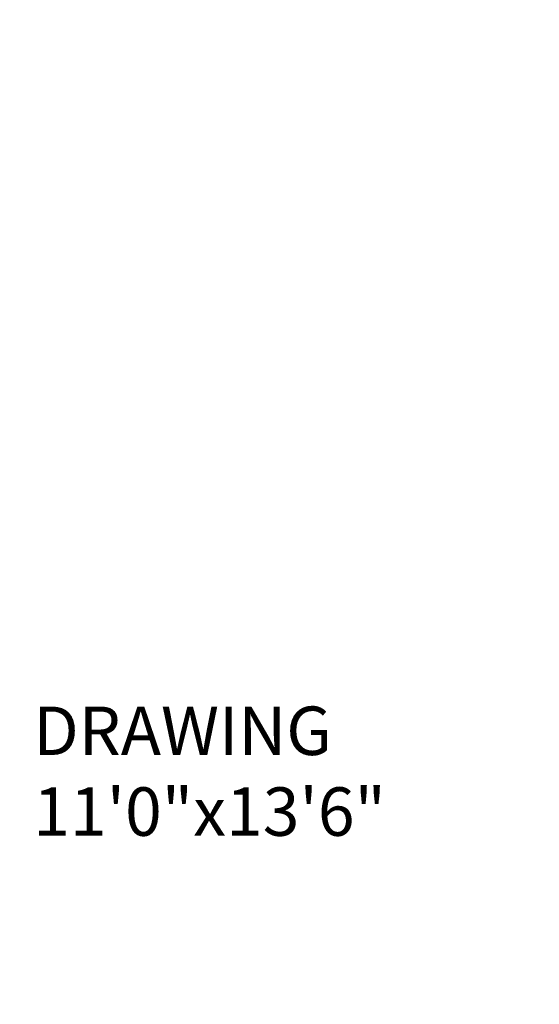
# Model space of a CAD drawing. Units: inches. Extents: x 963 to 2075, y 289 to 2657.
# Tile 18 of 98: x 1403 to 1457, y 1718 to 1820. Entities that reach past the tile are written whole.
import ezdxf

# ---------------------------------------------------------------- set-up
doc = ezdxf.new("R2010")
doc.units = ezdxf.units.IN
doc.layers.add('A-AREA-IDEN', color=7, linetype='Continuous', lineweight=18)
doc.layers.add('A-WALL-PATT', color=8, linetype='Continuous', lineweight=13)
doc.styles.get("Standard").update_dxf_attribs({"font": 'arial.ttf'})

msp = doc.modelspace()

# ---------------------------------------------------------------- hatches: boundary and pattern name
at = {"layer": 'A-WALL-PATT'}
h = msp.add_hatch(dxfattribs=at)
h.set_pattern_fill('ANSI32', color=256)
h.paths.add_polyline_path([(1296.92, 2558.32), (1203.92, 2558.32), (1203.92, 2493.82), (1191.53, 2493.82), (1191.53, 2489.32), (1211.06, 2489.32), (1211.06, 2492.02), (1211.06, 2493.82), (1208.42, 2493.82), (1208.42, 2553.82), (1292.42, 2553.82), (1292.42, 2538.86), (1296.92, 2538.86)])
h.paths.add_polyline_path([(1442.42, 2558.32), (1349.42, 2558.32), (1349.42, 2538.94), (1353.92, 2538.94), (1353.92, 2553.82), (1437.92, 2553.82), (1437.92, 2493.82), (1434.54, 2493.82), (1434.54, 2489.32), (1448.31, 2489.32), (1448.31, 2491.57), (1448.31, 2493.82), (1442.42, 2493.82)])
h.paths.add_polyline_path([(1415.55, 2491.57), (1415.55, 2493.82), (1340.94, 2493.82), (1340.94, 2489.32), (1371.92, 2489.32), (1371.92, 2378.32), (1367.6, 2378.32), (1367.6, 2373.82), (1371.92, 2373.82), (1371.92, 2355.19), (1376.42, 2355.19), (1376.42, 2489.32), (1415.55, 2489.32)])
h.paths.add_polyline_path([(1304.94, 2491.57), (1304.94, 2493.82), (1296.92, 2493.82), (1296.92, 2514.86), (1292.42, 2514.86), (1292.42, 2493.82), (1232.81, 2493.82), (1232.81, 2489.32), (1256.42, 2489.32), (1256.42, 2327.32), (1253.71, 2327.32), (1253.71, 2322.82), (1328.42, 2322.82), (1328.42, 2331.15), (1323.92, 2331.15), (1323.92, 2327.32), (1260.92, 2327.32), (1260.92, 2373.82), (1323.92, 2373.82), (1323.92, 2357.81), (1328.42, 2357.81), (1328.42, 2373.82), (1346.01, 2373.82), (1346.01, 2376.07), (1346.01, 2378.32), (1260.92, 2378.32), (1260.92, 2489.32), (1304.94, 2489.32)])
h.paths.add_polyline_path([(1226.65, 2327.32), (1124.42, 2327.32), (1124.42, 2347.45), (1119.92, 2347.45), (1119.92, 2322.82), (1163.42, 2322.82), (1163.42, 2305.43), (1165.67, 2305.43), (1167.92, 2305.43), (1167.92, 2322.82), (1226.65, 2322.82), (1226.65, 2325.07)])
h.paths.add_polyline_path([(1095.92, 2489.32), (1124.42, 2489.32), (1131.53, 2489.32), (1131.53, 2491.57), (1131.53, 2493.82), (1119.92, 2493.82), (1091.42, 2493.82), (1091.42, 2417.32), (1095.92, 2417.32), (1119.92, 2417.32), (1119.92, 2407.45), (1124.42, 2407.45), (1124.42, 2421.82), (1095.92, 2421.82)])
h.paths.add_polyline_path([(1512.92, 2558.32), (1508.42, 2558.32), (1508.42, 2493.82), (1503.4, 2493.82), (1503.4, 2489.32), (1508.42, 2489.32), (1508.42, 2327.32), (1376.42, 2327.32), (1376.42, 2330.27), (1371.92, 2330.27), (1371.92, 2298.74), (1376.42, 2298.74), (1376.42, 2322.82), (1508.42, 2322.82), (1508.42, 2165.32), (1504.26, 2165.32), (1504.26, 2160.82), (1508.42, 2160.82), (1508.42, 2108.32), (1512.92, 2108.32), (1512.92, 2160.82), (1516.18, 2160.82), (1516.18, 2163.07), (1516.18, 2165.32), (1512.92, 2165.32), (1512.92, 2322.82), (1644.92, 2322.82), (1644.92, 2298.74), (1649.42, 2298.74), (1649.42, 2322.82), (1649.42, 2330.94), (1647.17, 2330.94), (1644.92, 2330.94), (1644.92, 2327.32), (1512.92, 2327.32), (1512.92, 2489.32), (1516.76, 2489.32), (1516.76, 2491.57), (1516.76, 2493.82), (1512.92, 2493.82)])
h.paths.add_polyline_path([(1671.92, 2558.32), (1578.92, 2558.32), (1578.92, 2493.82), (1573.53, 2493.82), (1573.53, 2489.32), (1586.54, 2489.32), (1586.54, 2491.57), (1586.54, 2493.82), (1583.42, 2493.82), (1583.42, 2553.82), (1667.42, 2553.82), (1667.42, 2541.11), (1671.92, 2541.11)])
h.paths.add_polyline_path([(1681.26, 2493.82), (1671.92, 2493.82), (1671.92, 2517.11), (1667.42, 2517.11), (1667.42, 2493.82), (1610.22, 2493.82), (1610.22, 2489.32), (1644.92, 2489.32), (1644.92, 2357.87), (1649.42, 2357.87), (1649.42, 2373.82), (1652.2, 2373.82), (1652.2, 2375.83), (1652.2, 2378.32), (1649.42, 2378.32), (1649.42, 2489.32), (1681.26, 2489.32), (1681.26, 2491.57)])
h.paths.add_polyline_path([(1821.92, 2558.32), (1728.92, 2558.32), (1728.92, 2541), (1733.42, 2541), (1733.42, 2553.82), (1817.42, 2553.82), (1817.42, 2493.82), (1813.51, 2493.82), (1813.51, 2489.32), (1830.08, 2489.32), (1830.08, 2491.57), (1830.08, 2493.82), (1821.92, 2493.82)])
h.paths.add_polyline_path([(1794.24, 2493.82), (1717.26, 2493.82), (1717.26, 2489.32), (1760.42, 2489.32), (1760.42, 2378.32), (1674.4, 2378.32), (1674.4, 2373.82), (1692.92, 2373.82), (1692.92, 2356.95), (1697.42, 2356.95), (1697.42, 2373.82), (1760.42, 2373.82), (1760.42, 2327.32), (1697.42, 2327.32), (1697.42, 2333.34), (1692.92, 2333.34), (1692.92, 2322.82), (1768.04, 2322.82), (1768.04, 2325.07), (1768.04, 2327.32), (1764.92, 2327.32), (1764.92, 2489.32), (1794.24, 2489.32)])
h.paths.add_polyline_path([(1733.42, 2517), (1728.92, 2517), (1728.92, 2493.82), (1733.42, 2493.82)], flags=17)
h.paths.add_polyline_path([(1929.92, 2493.82), (1890.08, 2493.82), (1890.08, 2489.32), (1896.92, 2489.32), (1925.42, 2489.32), (1925.42, 2421.82), (1896.92, 2421.82), (1896.92, 2408.32), (1901.42, 2408.32), (1901.42, 2417.32), (1925.42, 2417.32), (1929.92, 2417.32)])
h.paths.add_polyline_path([(1901.42, 2348.32), (1896.92, 2348.32), (1896.92, 2327.32), (1800.42, 2327.32), (1800.42, 2322.82), (1853.42, 2322.82), (1853.42, 2309.45), (1857.92, 2309.45), (1857.92, 2322.82), (1901.42, 2322.82)])
h.paths.add_polyline_path([(1857.92, 2249.45), (1853.42, 2249.45), (1853.42, 2214.82), (1686.31, 2214.82), (1686.31, 2210.32), (1853.42, 2210.32), (1853.42, 2202.13), (1857.92, 2202.13), (1857.92, 2210.32)])
h.paths.add_polyline_path([(1857.92, 2142.13), (1853.42, 2142.13), (1853.42, 2115.42), (1841.42, 2115.42), (1841.42, 2088.53), (1841.42, 2046.95), (1845.92, 2046.95), (1845.92, 2110.92), (1905.92, 2110.92), (1905.92, 2092.52), (1910.42, 2092.52), (1910.42, 2115.42), (1857.92, 2115.42)])
h.paths.add_polyline_path([(1532.44, 1482.34), (1573.46, 1482.34), (1573.46, 1501), (1532.44, 1501)], flags=9)
h.paths.add_polyline_path([(1438.66, 1486.3), (1479.68, 1486.3), (1479.68, 1504.96), (1438.66, 1504.96)], flags=9)
h.paths.add_polyline_path([(1411.22, 1365.31), (1659.14, 1365.31), (1659.14, 1402.4), (1411.22, 1402.4)], flags=9)
h.paths.add_polyline_path([(1185.67, 2296.3), (1248.16, 2296.3), (1248.16, 2314.95), (1185.67, 2314.95)], flags=9)
h.paths.add_polyline_path([(1177.31, 2187.35), (1216.15, 2187.35), (1216.15, 2206.01), (1177.31, 2206.01)], flags=9)
h.paths.add_polyline_path([(1295.1, 1602.08), (1328.26, 1602.08), (1328.26, 1620.74), (1295.1, 1620.74)], flags=9)
h.paths.add_polyline_path([(1525.13, 2005.99), (1558.39, 2005.99), (1558.39, 2024.65), (1525.13, 2024.65)], flags=9)
h.paths.add_polyline_path([(1459.61, 1977.13), (1472.19, 1977.13), (1472.19, 1987.43), (1459.61, 1987.43)], flags=9)
h.paths.add_polyline_path([(1467.81, 2053.68), (1480.02, 2053.68), (1480.02, 2063.98), (1467.81, 2063.98)], flags=9)
h.paths.add_polyline_path([(1555.18, 2119.02), (1584.56, 2119.02), (1584.56, 2137.68), (1555.18, 2137.68)], flags=25)
h.paths.add_polyline_path([(1405.39, 2115.29), (1444.48, 2115.29), (1444.48, 2133.95), (1405.39, 2133.95)], flags=25)
h.paths.add_polyline_path([(1698.48, 2004.26), (1727.69, 2004.26), (1727.69, 2022.92), (1698.48, 2022.92)], flags=9)
h.paths.add_polyline_path([(1612.16, 1972.86), (1629.02, 1972.86), (1629.02, 1983.16), (1612.16, 1983.16)], flags=9)
h.paths.add_polyline_path([(1608.29, 2060.04), (1625.15, 2060.04), (1625.15, 2070.34), (1608.29, 2070.34)], flags=9)
h.paths.add_polyline_path([(1527.95, 1684.4), (1566.79, 1684.4), (1566.79, 1703.06), (1527.95, 1703.06)], flags=9)
h.paths.add_polyline_path([(1422.79, 1683.59), (1461.63, 1683.59), (1461.63, 1702.25), (1422.79, 1702.25)], flags=9)
h.paths.add_polyline_path([(1531.26, 1732.46), (1574.01, 1732.46), (1574.01, 1751.12), (1531.26, 1751.12)], flags=9)
h.paths.add_polyline_path([(1402.87, 1732.85), (1439.8, 1732.85), (1439.8, 1751.5), (1402.87, 1751.5)], flags=9)
h.paths.add_polyline_path([(1243.12, 1923.13), (1281.96, 1923.13), (1281.96, 1941.79), (1243.12, 1941.79)], flags=9)
h.paths.add_polyline_path([(1181.75, 1792.27), (1244.24, 1792.27), (1244.24, 1810.93), (1181.75, 1810.93)], flags=9)
h.paths.add_polyline_path([(1265.82, 1670.3), (1316.07, 1670.3), (1316.07, 1688.96), (1265.82, 1688.96)], flags=9)
h.paths.add_polyline_path([(1140.26, 1676.05), (1179.1, 1676.05), (1179.1, 1694.71), (1140.26, 1694.71)], flags=9)
h.paths.add_polyline_path([(1107.49, 1490.89), (1143.37, 1490.89), (1143.37, 1509.55), (1107.49, 1509.55)], flags=9)
h.paths.add_polyline_path([(1217.58, 1483.9), (1246.74, 1483.9), (1246.74, 1502.56), (1217.58, 1502.56)], flags=9)
h.paths.add_polyline_path([(1389.21, 1486.92), (1418.37, 1486.92), (1418.37, 1505.58), (1389.21, 1505.58)], flags=9)
h.paths.add_polyline_path([(1672.21, 1602.08), (1705.37, 1602.08), (1705.37, 1620.74), (1672.21, 1620.74)], flags=9)
h.paths.add_polyline_path([(1752.08, 1522.64), (1781.24, 1522.64), (1781.24, 1541.3), (1752.08, 1541.3)], flags=9)
h.paths.add_polyline_path([(1848.27, 1491.26), (1884.16, 1491.26), (1884.16, 1509.92), (1848.27, 1509.92)], flags=9)
h.paths.add_polyline_path([(1822.47, 1685.62), (1861.31, 1685.62), (1861.31, 1704.28), (1822.47, 1704.28)], flags=9)
h.paths.add_polyline_path([(1713.19, 1672.23), (1763.44, 1672.23), (1763.44, 1690.89), (1713.19, 1690.89)], flags=9)
h.paths.add_polyline_path([(1736.62, 1790.58), (1799.11, 1790.58), (1799.11, 1809.24), (1736.62, 1809.24)], flags=9)
h.paths.add_polyline_path([(1691.49, 1916.36), (1730.33, 1916.36), (1730.33, 1935.01), (1691.49, 1935.01)], flags=9)
h.paths.add_polyline_path([(1764.87, 1973.92), (1794.31, 1973.92), (1794.31, 1992.58), (1764.87, 1992.58)], flags=9)
h.paths.add_polyline_path([(1767.85, 2034.02), (1797.29, 2034.02), (1797.29, 2052.67), (1767.85, 2052.67)], flags=9)
h.paths.add_polyline_path([(1851.59, 2060.33), (1880.75, 2060.33), (1880.75, 2078.99), (1851.59, 2078.99)], flags=25)
h.paths.add_polyline_path([(1688.49, 2086.87), (1727.33, 2086.87), (1727.33, 2105.53), (1688.49, 2105.53)], flags=9)
h.paths.add_polyline_path([(1537.74, 2293.58), (1580.49, 2293.58), (1580.49, 2312.24), (1537.74, 2312.24)], flags=25)
h.paths.add_polyline_path([(1425.59, 2296.11), (1468.34, 2296.11), (1468.34, 2314.77), (1425.59, 2314.77)], flags=25)
h.paths.add_polyline_path([(1278.52, 2004.18), (1307.72, 2004.18), (1307.72, 2022.84), (1278.52, 2022.84)], flags=9)
h.paths.add_polyline_path([(1193.28, 1973.63), (1222.72, 1973.63), (1222.72, 1992.29), (1193.28, 1992.29)], flags=9)
h.paths.add_polyline_path([(1192.41, 2040.58), (1221.84, 2040.58), (1221.84, 2059.23), (1192.41, 2059.23)], flags=9)
h.paths.add_polyline_path([(1130.6, 1951.39), (1159.76, 1951.39), (1159.76, 1970.05), (1130.6, 1970.05)], flags=9)
h.paths.add_polyline_path([(1132.83, 2052.49), (1161.98, 2052.49), (1161.98, 2071.15), (1132.83, 2071.15)], flags=9)
h.paths.add_polyline_path([(1265.13, 2334.62), (1315.38, 2334.62), (1315.38, 2353.28), (1265.13, 2353.28)], flags=25)
h.paths.add_polyline_path([(1136.74, 2330.79), (1175.58, 2330.79), (1175.58, 2349.44), (1136.74, 2349.44)], flags=9)
h.paths.add_polyline_path([(1287.42, 2417.2), (1320.58, 2417.2), (1320.58, 2435.86), (1287.42, 2435.86)], flags=25)
h.paths.add_polyline_path([(1430.99, 2329.16), (1469.83, 2329.16), (1469.83, 2347.82), (1430.99, 2347.82)], flags=25)
h.paths.add_polyline_path([(1525.42, 2329.21), (1564.26, 2329.21), (1564.26, 2347.87), (1525.42, 2347.87)], flags=25)
h.paths.add_polyline_path([(1684.52, 2382.8), (1717.68, 2382.8), (1717.68, 2401.46), (1684.52, 2401.46)], flags=25)
h.paths.add_polyline_path([(1704.81, 2340.29), (1755.05, 2340.29), (1755.05, 2358.95), (1704.81, 2358.95)], flags=25)
h.paths.add_polyline_path([(1694.11, 2287.76), (1756.6, 2287.76), (1756.6, 2306.41), (1694.11, 2306.41)], flags=9)
h.paths.add_polyline_path([(1815.78, 2329.86), (1854.62, 2329.86), (1854.62, 2348.52), (1815.78, 2348.52)], flags=9)
h.paths.add_polyline_path([(1842.87, 2514.26), (1878.76, 2514.26), (1878.76, 2532.91), (1842.87, 2532.91)], flags=9)
h.paths.add_polyline_path([(1769.51, 2531.45), (1798.67, 2531.45), (1798.67, 2550.1), (1769.51, 2550.1)], flags=25)
h.paths.add_polyline_path([(1594.77, 2518.47), (1623.93, 2518.47), (1623.93, 2537.13), (1594.77, 2537.13)], flags=25)
h.paths.add_polyline_path([(1520.72, 2516.18), (1556.61, 2516.18), (1556.61, 2534.84), (1520.72, 2534.84)], flags=25)
h.paths.add_polyline_path([(1464.46, 2516.69), (1500.34, 2516.69), (1500.34, 2535.35), (1464.46, 2535.35)], flags=25)
h.paths.add_polyline_path([(1365.7, 2528.97), (1394.85, 2528.97), (1394.85, 2547.63), (1365.7, 2547.63)], flags=25)
h.paths.add_polyline_path([(1222.84, 2516.23), (1252, 2516.23), (1252, 2534.89), (1222.84, 2534.89)], flags=25)
h.paths.add_polyline_path([(1104.55, 2509.6), (1140.43, 2509.6), (1140.43, 2528.26), (1104.55, 2528.26)], flags=9)
h = msp.add_hatch(dxfattribs=at)
h.set_pattern_fill('ANSI32', color=256)
h.paths.add_polyline_path([(1335.97, 2212.57), (1335.97, 2214.82), (1167.92, 2214.82), (1167.92, 2245.43), (1163.42, 2245.43), (1163.42, 2210.32), (1163.42, 2194.81), (1167.92, 2194.81), (1167.92, 2210.32), (1335.97, 2210.32)])
h.paths.add_polyline_path([(1532.44, 1482.34), (1573.46, 1482.34), (1573.46, 1501), (1532.44, 1501)], flags=9)
h.paths.add_polyline_path([(1438.66, 1486.3), (1479.68, 1486.3), (1479.68, 1504.96), (1438.66, 1504.96)], flags=9)
h.paths.add_polyline_path([(1411.22, 1365.31), (1659.14, 1365.31), (1659.14, 1402.4), (1411.22, 1402.4)], flags=9)
h.paths.add_polyline_path([(1185.67, 2296.3), (1248.16, 2296.3), (1248.16, 2314.95), (1185.67, 2314.95)], flags=9)
h.paths.add_polyline_path([(1177.31, 2187.35), (1216.15, 2187.35), (1216.15, 2206.01), (1177.31, 2206.01)], flags=9)
h.paths.add_polyline_path([(1295.1, 1602.08), (1328.26, 1602.08), (1328.26, 1620.74), (1295.1, 1620.74)], flags=9)
h.paths.add_polyline_path([(1525.13, 2005.99), (1558.39, 2005.99), (1558.39, 2024.65), (1525.13, 2024.65)], flags=9)
h.paths.add_polyline_path([(1459.61, 1977.13), (1472.19, 1977.13), (1472.19, 1987.43), (1459.61, 1987.43)], flags=9)
h.paths.add_polyline_path([(1467.81, 2053.68), (1480.02, 2053.68), (1480.02, 2063.98), (1467.81, 2063.98)], flags=9)
h.paths.add_polyline_path([(1555.18, 2119.02), (1584.56, 2119.02), (1584.56, 2137.68), (1555.18, 2137.68)], flags=9)
h.paths.add_polyline_path([(1405.39, 2115.29), (1444.48, 2115.29), (1444.48, 2133.95), (1405.39, 2133.95)], flags=9)
h.paths.add_polyline_path([(1698.48, 2004.26), (1727.69, 2004.26), (1727.69, 2022.92), (1698.48, 2022.92)], flags=9)
h.paths.add_polyline_path([(1612.16, 1972.86), (1629.02, 1972.86), (1629.02, 1983.16), (1612.16, 1983.16)], flags=9)
h.paths.add_polyline_path([(1608.29, 2060.04), (1625.15, 2060.04), (1625.15, 2070.34), (1608.29, 2070.34)], flags=9)
h.paths.add_polyline_path([(1527.95, 1684.4), (1566.79, 1684.4), (1566.79, 1703.06), (1527.95, 1703.06)], flags=9)
h.paths.add_polyline_path([(1422.79, 1683.59), (1461.63, 1683.59), (1461.63, 1702.25), (1422.79, 1702.25)], flags=9)
h.paths.add_polyline_path([(1531.26, 1732.46), (1574.01, 1732.46), (1574.01, 1751.12), (1531.26, 1751.12)], flags=9)
h.paths.add_polyline_path([(1402.87, 1732.85), (1439.8, 1732.85), (1439.8, 1751.5), (1402.87, 1751.5)], flags=9)
h.paths.add_polyline_path([(1243.12, 1923.13), (1281.96, 1923.13), (1281.96, 1941.79), (1243.12, 1941.79)], flags=9)
h.paths.add_polyline_path([(1181.75, 1792.27), (1244.24, 1792.27), (1244.24, 1810.93), (1181.75, 1810.93)], flags=9)
h.paths.add_polyline_path([(1265.82, 1670.3), (1316.07, 1670.3), (1316.07, 1688.96), (1265.82, 1688.96)], flags=9)
h.paths.add_polyline_path([(1140.26, 1676.05), (1179.1, 1676.05), (1179.1, 1694.71), (1140.26, 1694.71)], flags=9)
h.paths.add_polyline_path([(1107.49, 1490.89), (1143.37, 1490.89), (1143.37, 1509.55), (1107.49, 1509.55)], flags=9)
h.paths.add_polyline_path([(1217.58, 1483.9), (1246.74, 1483.9), (1246.74, 1502.56), (1217.58, 1502.56)], flags=9)
h.paths.add_polyline_path([(1389.21, 1486.92), (1418.37, 1486.92), (1418.37, 1505.58), (1389.21, 1505.58)], flags=9)
h.paths.add_polyline_path([(1672.21, 1602.08), (1705.37, 1602.08), (1705.37, 1620.74), (1672.21, 1620.74)], flags=9)
h.paths.add_polyline_path([(1752.08, 1522.64), (1781.24, 1522.64), (1781.24, 1541.3), (1752.08, 1541.3)], flags=9)
h.paths.add_polyline_path([(1848.27, 1491.26), (1884.16, 1491.26), (1884.16, 1509.92), (1848.27, 1509.92)], flags=9)
h.paths.add_polyline_path([(1822.47, 1685.62), (1861.31, 1685.62), (1861.31, 1704.28), (1822.47, 1704.28)], flags=9)
h.paths.add_polyline_path([(1713.19, 1672.23), (1763.44, 1672.23), (1763.44, 1690.89), (1713.19, 1690.89)], flags=9)
h.paths.add_polyline_path([(1736.62, 1790.58), (1799.11, 1790.58), (1799.11, 1809.24), (1736.62, 1809.24)], flags=9)
h.paths.add_polyline_path([(1691.49, 1916.36), (1730.33, 1916.36), (1730.33, 1935.01), (1691.49, 1935.01)], flags=9)
h.paths.add_polyline_path([(1764.87, 1973.92), (1794.31, 1973.92), (1794.31, 1992.58), (1764.87, 1992.58)], flags=9)
h.paths.add_polyline_path([(1767.85, 2034.02), (1797.29, 2034.02), (1797.29, 2052.67), (1767.85, 2052.67)], flags=9)
h.paths.add_polyline_path([(1851.59, 2060.33), (1880.75, 2060.33), (1880.75, 2078.99), (1851.59, 2078.99)], flags=9)
h.paths.add_polyline_path([(1688.49, 2086.87), (1727.33, 2086.87), (1727.33, 2105.53), (1688.49, 2105.53)], flags=9)
h.paths.add_polyline_path([(1537.74, 2293.58), (1580.49, 2293.58), (1580.49, 2312.24), (1537.74, 2312.24)], flags=9)
h.paths.add_polyline_path([(1425.59, 2296.11), (1468.34, 2296.11), (1468.34, 2314.77), (1425.59, 2314.77)], flags=9)
h.paths.add_polyline_path([(1278.52, 2004.18), (1307.72, 2004.18), (1307.72, 2022.84), (1278.52, 2022.84)], flags=9)
h.paths.add_polyline_path([(1193.28, 1973.63), (1222.72, 1973.63), (1222.72, 1992.29), (1193.28, 1992.29)], flags=9)
h.paths.add_polyline_path([(1192.41, 2040.58), (1221.84, 2040.58), (1221.84, 2059.23), (1192.41, 2059.23)], flags=9)
h.paths.add_polyline_path([(1130.6, 1951.39), (1159.76, 1951.39), (1159.76, 1970.05), (1130.6, 1970.05)], flags=9)
h.paths.add_polyline_path([(1132.83, 2052.49), (1161.98, 2052.49), (1161.98, 2071.15), (1132.83, 2071.15)], flags=9)
h.paths.add_polyline_path([(1265.13, 2334.62), (1315.38, 2334.62), (1315.38, 2353.28), (1265.13, 2353.28)], flags=9)
h.paths.add_polyline_path([(1136.74, 2330.79), (1175.58, 2330.79), (1175.58, 2349.44), (1136.74, 2349.44)], flags=9)
h.paths.add_polyline_path([(1287.42, 2417.2), (1320.58, 2417.2), (1320.58, 2435.86), (1287.42, 2435.86)], flags=9)
h.paths.add_polyline_path([(1430.99, 2329.16), (1469.83, 2329.16), (1469.83, 2347.82), (1430.99, 2347.82)], flags=9)
h.paths.add_polyline_path([(1525.42, 2329.21), (1564.26, 2329.21), (1564.26, 2347.87), (1525.42, 2347.87)], flags=9)
h.paths.add_polyline_path([(1684.52, 2382.8), (1717.68, 2382.8), (1717.68, 2401.46), (1684.52, 2401.46)], flags=9)
h.paths.add_polyline_path([(1704.81, 2340.29), (1755.05, 2340.29), (1755.05, 2358.95), (1704.81, 2358.95)], flags=9)
h.paths.add_polyline_path([(1694.11, 2287.76), (1756.6, 2287.76), (1756.6, 2306.41), (1694.11, 2306.41)], flags=9)
h.paths.add_polyline_path([(1815.78, 2329.86), (1854.62, 2329.86), (1854.62, 2348.52), (1815.78, 2348.52)], flags=9)
h.paths.add_polyline_path([(1842.87, 2514.26), (1878.76, 2514.26), (1878.76, 2532.91), (1842.87, 2532.91)], flags=9)
h.paths.add_polyline_path([(1769.51, 2531.45), (1798.67, 2531.45), (1798.67, 2550.1), (1769.51, 2550.1)], flags=9)
h.paths.add_polyline_path([(1594.77, 2518.47), (1623.93, 2518.47), (1623.93, 2537.13), (1594.77, 2537.13)], flags=9)
h.paths.add_polyline_path([(1520.72, 2516.18), (1556.61, 2516.18), (1556.61, 2534.84), (1520.72, 2534.84)], flags=9)
h.paths.add_polyline_path([(1464.46, 2516.69), (1500.34, 2516.69), (1500.34, 2535.35), (1464.46, 2535.35)], flags=9)
h.paths.add_polyline_path([(1365.7, 2528.97), (1394.85, 2528.97), (1394.85, 2547.63), (1365.7, 2547.63)], flags=9)
h.paths.add_polyline_path([(1222.84, 2516.23), (1252, 2516.23), (1252, 2534.89), (1222.84, 2534.89)], flags=9)
h.paths.add_polyline_path([(1104.55, 2509.6), (1140.43, 2509.6), (1140.43, 2528.26), (1104.55, 2528.26)], flags=9)

# ---------------------------------------------------------------- texts
at = {"layer": 'A-AREA-IDEN', "insert": (1404.88, 1749.01), "char_height": 5, "attachment_point": 1}
msp.add_mtext_dynamic_manual_height_columns('DRAWING\\P11\'0"x13\'6"', width=142.7562, gutter_width=12.5, heights=[0], dxfattribs=at)

doc.saveas('drawing.dxf')
